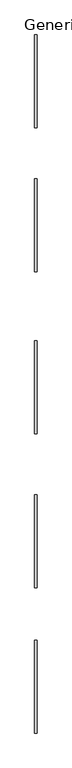
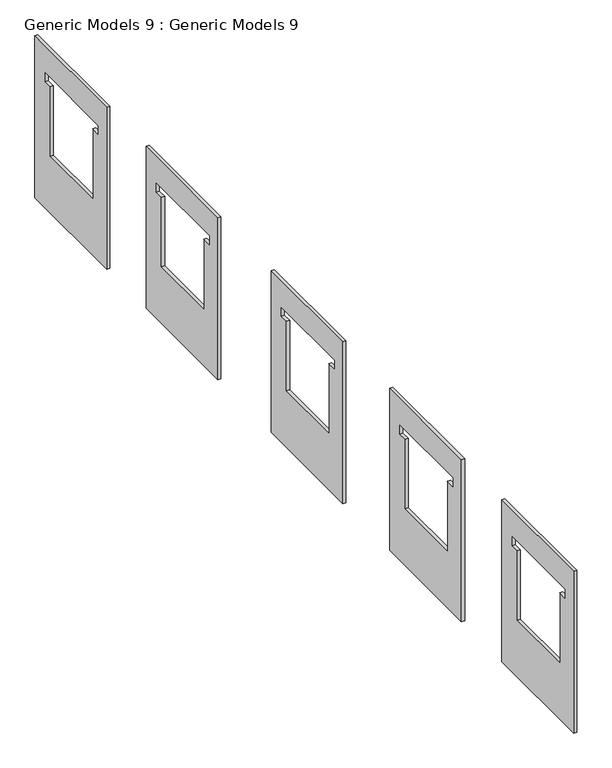
"""IFC4 building model written with IfcOpenShell, lengths in millimetres: proxy geometry, Generic Models 9 : Generic Models 9."""

from ifc_helpers import new_model, si_unit, frame, origin, place, context, project, spatial, polyline, outline, extrude, source, transform, mapped, element, save


def generic_models_9_generic_models_9_b0d80d45(model_context):
    return source(origin(), model_context, "Body", "SweptSolid", [
        extrude(outline(polyline([(-4116.6073314, 6198.4771746), (-4116.6073314, 3352.8), (-6184.571691, 3352.8), (-6184.571691, 6198.4771746), (-4116.6073314, 6198.4771746)]), holes=[polyline([(-4408.7073314, 5724.4), (-5932.7073314, 5724.4), (-5932.7073314, 5572.0), (-5780.3073314, 5572.0), (-5780.3073314, 4352.8), (-4561.1073314, 4352.8), (-4561.1073314, 5572.0), (-4408.7073314, 5572.0), (-4408.7073314, 5724.4)])]), frame((10137.9423568, 0.0, 0.0), z_axis=(1.0, 0.0, 0.0), x_axis=(0.0, 1.0, 0.0)), (0.0, 0.0, 1.0), 50.8),
        extrude(outline(polyline([(-884.4573314, 6198.4771746), (-884.4573314, 3352.8), (-2952.421691, 3352.8), (-2952.421691, 6198.4771746), (-884.4573314, 6198.4771746)]), holes=[polyline([(-1176.5573314, 5724.4), (-2700.5573314, 5724.4), (-2700.5573314, 5572.0), (-2548.1573314, 5572.0), (-2548.1573314, 4352.8), (-1328.9573314, 4352.8), (-1328.9573314, 5572.0), (-1176.5573314, 5572.0), (-1176.5573314, 5724.4)])]), frame((10137.9423568, 0.0, 0.0), z_axis=(1.0, 0.0, 0.0), x_axis=(0.0, 1.0, 0.0)), (0.0, 0.0, 1.0), 50.8),
        extrude(outline(polyline([(2531.8426686, 6198.4771746), (2531.8426686, 3352.8), (463.878309, 3352.8), (463.878309, 6198.4771746), (2531.8426686, 6198.4771746)]), holes=[polyline([(2239.7426686, 5724.4), (715.7426686, 5724.4), (715.7426686, 5572.0), (868.1426686, 5572.0), (868.1426686, 4352.8), (2087.3426686, 4352.8), (2087.3426686, 5572.0), (2239.7426686, 5572.0), (2239.7426686, 5724.4)])]), frame((10137.9423568, 0.0, 0.0), z_axis=(1.0, 0.0, 0.0), x_axis=(0.0, 1.0, 0.0)), (0.0, 0.0, 1.0), 50.8),
        extrude(outline(polyline([(6132.2926686, 6198.4771746), (6132.2926686, 3352.8), (4064.328309, 3352.8), (4064.328309, 6198.4771746), (6132.2926686, 6198.4771746)]), holes=[polyline([(5840.1926686, 5724.4), (4316.1926686, 5724.4), (4316.1926686, 5572.0), (4468.5926686, 5572.0), (4468.5926686, 4352.8), (5687.7926686, 4352.8), (5687.7926686, 5572.0), (5840.1926686, 5572.0), (5840.1926686, 5724.4)])]), frame((10137.9423568, 0.0, 0.0), z_axis=(1.0, 0.0, 0.0), x_axis=(0.0, 1.0, 0.0)), (0.0, 0.0, 1.0), 50.8),
        extrude(outline(polyline([(9332.6926686, 6198.4771746), (9332.6926686, 3352.8), (7264.728309, 3352.8), (7264.728309, 6198.4771746), (9332.6926686, 6198.4771746)]), holes=[polyline([(9040.5926686, 5724.4), (7516.5926686, 5724.4), (7516.5926686, 5572.0), (7668.9926686, 5572.0), (7668.9926686, 4352.8), (8888.1926686, 4352.8), (8888.1926686, 5572.0), (9040.5926686, 5572.0), (9040.5926686, 5724.4)])]), frame((10137.9423568, 0.0, 0.0), z_axis=(1.0, 0.0, 0.0), x_axis=(0.0, 1.0, 0.0)), (0.0, 0.0, 1.0), 50.8),
    ])


if __name__ == "__main__":
    model = new_model("IFC4")
    model_context = context("Model", 3, world=origin())
    ifc_project = project(units=[si_unit("LENGTHUNIT", "METRE", prefix="MILLI")], contexts=[model_context])
    site = spatial("IfcSite", under=ifc_project)
    building = spatial("IfcBuilding", under=site)
    placement = place(None, origin())
    generic_models_9_generic_models_9_shape = generic_models_9_generic_models_9_b0d80d45(model_context)
    element("IfcBuildingElementProxy", 1, Name="Generic Models 9 : Generic Models 9", ObjectType="Generic Models 9 : Generic Models 9", at=placement, inside=building, context=model_context, shape_type="MappedRepresentation", body=[
        mapped(generic_models_9_generic_models_9_shape, transform((0.0, 0.0, 0.0), x_axis=(1.0, 0.0, 0.0), y_axis=(0.0, 1.0, 0.0), z_axis=(0.0, 0.0, 1.0))),
    ])
    save(model, "model.ifc")

# Revit data of these elements
# Element 1 (IfcBuildingElementProxy, "Generic Models 9 : Generic Models 9")
#   Materials on its faces: "WOOD MATERIAL 9\""
# Materials
#   "WOOD MATERIAL 9\"": class "Generic", colour RGB 120 120 120, transparency 0, Cost = 0
